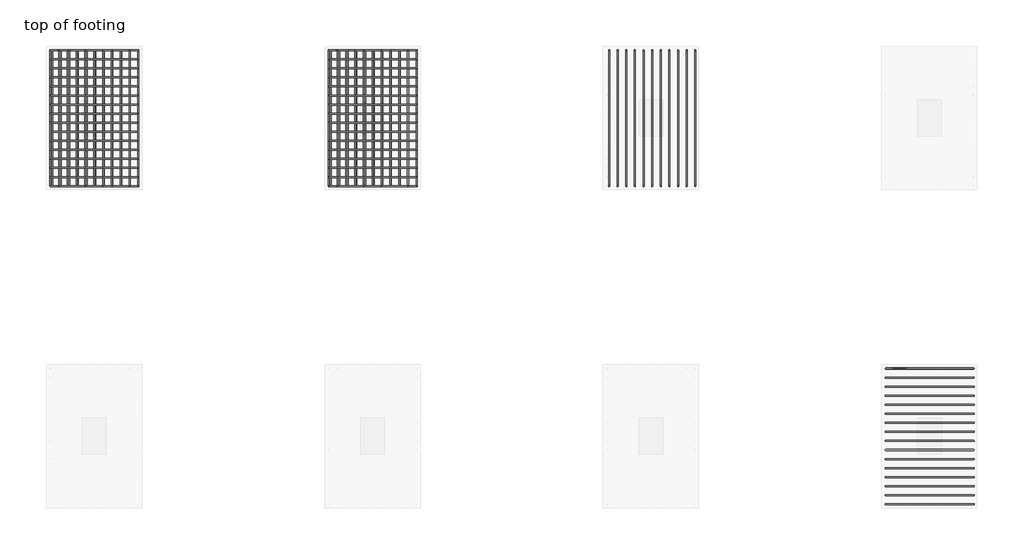
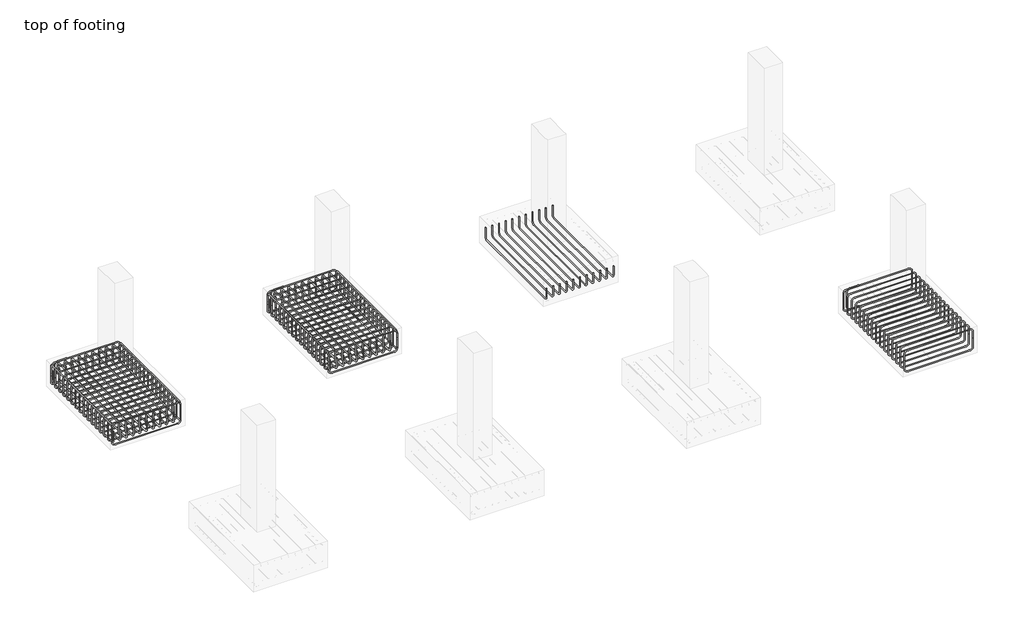
# One storey, part 6 of 8: 14 reinforcing bars.
"""IFC4 building model written with IfcOpenShell, lengths in millimetres."""

from ifc_helpers import new_model, si_unit, point, frame, origin, place, context, project, spatial, polyline, circle_curve, trimmed, segment, composite_curve, source, transform, mapped, element, save
from ifc_brep_helpers import swept_disk

model = new_model("IFC4")

# Units and contexts
model_context = context("Model", 3, world=origin())
ifc_project = project(units=[si_unit("LENGTHUNIT", "METRE", prefix="MILLI")], contexts=[model_context])

# Site, building, storey
site = spatial("IfcSite", under=ifc_project)
building = spatial("IfcBuilding", under=site)
storey = spatial("IfcBuildingStorey", under=building, Name="top of footing", Elevation=-1828.8)

# Reinforcing bars
placement = place(None, origin())
reinforcing_bar_shape = source(origin(), model_context, "Body", "SolidModel", [
    swept_disk(composite_curve([segment(polyline([(-10685.4300189, 16682.8075251, -2014.4920065), (-10685.4300189, 16682.8075251, -2161.7920065)]), True, "CONTINUOUS"), segment(trimmed(circle_curve(frame((-10685.4300189, 16729.1575251, -2161.7920065), z_axis=(1.0, 0.0, 0.0), x_axis=(0.0, -46.349999999998545, 0.0)), 46.35), [point((-10685.4300189, 16682.8075251, -2161.7920065))], [point((-10685.4300189, 16729.1575251, -2208.1420065))], True, "CARTESIAN"), True, "CONTINUOUS"), segment(polyline([(-10685.4300189, 16729.1575251, -2208.1420065), (-10685.4300189, 18343.7575251, -2208.1420065)]), True, "CONTINUOUS"), segment(trimmed(circle_curve(frame((-10685.4300189, 18343.7575251, -2161.7920065), z_axis=(1.0, 0.0, 0.0), x_axis=(0.0, 0.0, -46.350000000000364)), 46.35), [point((-10685.4300189, 18343.7575251, -2208.1420065))], [point((-10685.4300189, 18390.1075251, -2161.7920065))], True, "CARTESIAN"), True, "CONTINUOUS"), segment(polyline([(-10685.4300189, 18390.1075251, -2161.7920065), (-10685.4300189, 18390.1075251, -2014.4920065)]), True, "CONTINUOUS")], self_intersect=False), 6.35),
])
element("IfcReinforcingBar", 1, at=placement, inside=storey, context=model_context, shape_type="MappedRepresentation", body=[
    mapped(reinforcing_bar_shape, transform((0.0, 0.0, 0.0), x_axis=(1.0, 0.0, 0.0), y_axis=(0.0, 1.0, 0.0), z_axis=(0.0, 0.0, 1.0))),
    mapped(reinforcing_bar_shape, transform((-108.3645139, 0.0, 0.0), x_axis=(1.0, 0.0, 0.0), y_axis=(0.0, 1.0, 0.0), z_axis=(0.0, 0.0, 1.0))),
    mapped(reinforcing_bar_shape, transform((-216.7290279, 0.0, 0.0), x_axis=(1.0, 0.0, 0.0), y_axis=(0.0, 1.0, 0.0), z_axis=(0.0, 0.0, 1.0))),
    mapped(reinforcing_bar_shape, transform((-325.0935418, 0.0, 0.0), x_axis=(1.0, 0.0, 0.0), y_axis=(0.0, 1.0, 0.0), z_axis=(0.0, 0.0, 1.0))),
    mapped(reinforcing_bar_shape, transform((-433.4580557, 0.0, 0.0), x_axis=(1.0, 0.0, 0.0), y_axis=(0.0, 1.0, 0.0), z_axis=(0.0, 0.0, 1.0))),
    mapped(reinforcing_bar_shape, transform((-541.8225696, 0.0, 0.0), x_axis=(1.0, 0.0, 0.0), y_axis=(0.0, 1.0, 0.0), z_axis=(0.0, 0.0, 1.0))),
    mapped(reinforcing_bar_shape, transform((-650.1870836, 0.0, 0.0), x_axis=(1.0, 0.0, 0.0), y_axis=(0.0, 1.0, 0.0), z_axis=(0.0, 0.0, 1.0))),
    mapped(reinforcing_bar_shape, transform((-758.5515975, 0.0, 0.0), x_axis=(1.0, 0.0, 0.0), y_axis=(0.0, 1.0, 0.0), z_axis=(0.0, 0.0, 1.0))),
    mapped(reinforcing_bar_shape, transform((-866.9161114, 0.0, 0.0), x_axis=(1.0, 0.0, 0.0), y_axis=(0.0, 1.0, 0.0), z_axis=(0.0, 0.0, 1.0))),
    mapped(reinforcing_bar_shape, transform((-975.2806253, 0.0, 0.0), x_axis=(1.0, 0.0, 0.0), y_axis=(0.0, 1.0, 0.0), z_axis=(0.0, 0.0, 1.0))),
    mapped(reinforcing_bar_shape, transform((-1083.6451393, 0.0, 0.0), x_axis=(1.0, 0.0, 0.0), y_axis=(0.0, 1.0, 0.0), z_axis=(0.0, 0.0, 1.0))),
])
reinforcing_bar_2_shape = source(origin(), model_context, "Body", "SolidModel", [
    swept_disk(composite_curve([segment(polyline([(-11792.7300189, 16682.8075251, -2085.8010212), (-11792.7300189, 16682.8075251, -1938.5010212)]), True, "CONTINUOUS"), segment(trimmed(circle_curve(frame((-11792.7300189, 16729.1575251, -1938.5010212), z_axis=(-1.0, 0.0, 0.0), x_axis=(0.0, -46.349999999998545, 0.0)), 46.35), [point((-11792.7300189, 16682.8075251, -1938.5010212))], [point((-11792.7300189, 16729.1575251, -1892.1510212))], True, "CARTESIAN"), True, "CONTINUOUS"), segment(polyline([(-11792.7300189, 16729.1575251, -1892.1510212), (-11792.7300189, 18343.7575251, -1892.1510212)]), True, "CONTINUOUS"), segment(trimmed(circle_curve(frame((-11792.7300189, 18343.7575251, -1938.5010212), z_axis=(-1.0, 0.0, 0.0), x_axis=(0.0, 0.0, 46.34999999999991)), 46.35), [point((-11792.7300189, 18343.7575251, -1892.1510212))], [point((-11792.7300189, 18390.1075251, -1938.5010212))], True, "CARTESIAN"), True, "CONTINUOUS"), segment(polyline([(-11792.7300189, 18390.1075251, -1938.5010212), (-11792.7300189, 18390.1075251, -2085.8010212)]), True, "CONTINUOUS")], self_intersect=False), 6.35),
])
element("IfcReinforcingBar", 2, at=placement, inside=storey, context=model_context, shape_type="MappedRepresentation", body=[
    mapped(reinforcing_bar_2_shape, transform((0.0, 0.0, 0.0), x_axis=(1.0, 0.0, 0.0), y_axis=(0.0, 1.0, 0.0), z_axis=(0.0, 0.0, 1.0))),
    mapped(reinforcing_bar_2_shape, transform((110.73, 0.0, 0.0), x_axis=(1.0, 0.0, 0.0), y_axis=(0.0, 1.0, 0.0), z_axis=(0.0, 0.0, 1.0))),
    mapped(reinforcing_bar_2_shape, transform((221.46, 0.0, 0.0), x_axis=(1.0, 0.0, 0.0), y_axis=(0.0, 1.0, 0.0), z_axis=(0.0, 0.0, 1.0))),
    mapped(reinforcing_bar_2_shape, transform((332.19, 0.0, 0.0), x_axis=(1.0, 0.0, 0.0), y_axis=(0.0, 1.0, 0.0), z_axis=(0.0, 0.0, 1.0))),
    mapped(reinforcing_bar_2_shape, transform((442.92, 0.0, 0.0), x_axis=(1.0, 0.0, 0.0), y_axis=(0.0, 1.0, 0.0), z_axis=(0.0, 0.0, 1.0))),
    mapped(reinforcing_bar_2_shape, transform((553.65, 0.0, 0.0), x_axis=(1.0, 0.0, 0.0), y_axis=(0.0, 1.0, 0.0), z_axis=(0.0, 0.0, 1.0))),
    mapped(reinforcing_bar_2_shape, transform((664.38, 0.0, 0.0), x_axis=(1.0, 0.0, 0.0), y_axis=(0.0, 1.0, 0.0), z_axis=(0.0, 0.0, 1.0))),
    mapped(reinforcing_bar_2_shape, transform((775.11, 0.0, 0.0), x_axis=(1.0, 0.0, 0.0), y_axis=(0.0, 1.0, 0.0), z_axis=(0.0, 0.0, 1.0))),
    mapped(reinforcing_bar_2_shape, transform((885.84, 0.0, 0.0), x_axis=(1.0, 0.0, 0.0), y_axis=(0.0, 1.0, 0.0), z_axis=(0.0, 0.0, 1.0))),
    mapped(reinforcing_bar_2_shape, transform((996.57, 0.0, 0.0), x_axis=(1.0, 0.0, 0.0), y_axis=(0.0, 1.0, 0.0), z_axis=(0.0, 0.0, 1.0))),
    mapped(reinforcing_bar_2_shape, transform((1107.3, 0.0, 0.0), x_axis=(1.0, 0.0, 0.0), y_axis=(0.0, 1.0, 0.0), z_axis=(0.0, 0.0, 1.0))),
])
element("IfcReinforcingBar", 3, at=placement, inside=storey, context=model_context, shape_type="SolidModel", body=[
    swept_disk(composite_curve([segment(polyline([(-11543.0309105, 18390.1075251, -2232.45), (-11690.3309105, 18390.1075251, -2232.45)]), True, "CONTINUOUS"), segment(trimmed(circle_curve(frame((-11690.3309105, 18390.1075251, -2186.1), z_axis=(0.0, 1.0, 0.0), x_axis=(0.0, 0.0, -46.34999999999991)), 46.35), [point((-11690.3309105, 18390.1075251, -2232.45))], [point((-11736.6809105, 18390.1075251, -2186.1))], True, "CARTESIAN"), True, "CONTINUOUS"), segment(polyline([(-11736.6809105, 18390.1075251, -2186.1), (-11736.6809105, 18390.1075251, -1921.5)]), True, "CONTINUOUS"), segment(trimmed(circle_curve(frame((-11690.3309105, 18390.1075251, -1921.5), z_axis=(0.0, 1.0, 0.0), x_axis=(-46.349999999998545, 0.0, 0.0)), 46.35), [point((-11736.6809105, 18390.1075251, -1921.5))], [point((-11690.3309105, 18390.1075251, -1875.15))], True, "CARTESIAN"), True, "CONTINUOUS"), segment(polyline([(-11690.3309105, 18390.1075251, -1875.15), (-11543.0309105, 18390.1075251, -1875.15)]), True, "CONTINUOUS")], self_intersect=False), 6.35),
])
reinforcing_bar_3_shape = source(origin(), model_context, "Body", "SolidModel", [
    swept_disk(composite_curve([segment(polyline([(-10685.4300189, 18390.1075251, -2044.8290141), (-10685.4300189, 18390.1075251, -2192.1290141)]), True, "CONTINUOUS"), segment(trimmed(circle_curve(frame((-10731.7800189, 18390.1075251, -2192.1290141), z_axis=(0.0, 1.0, 0.0), x_axis=(46.350000000000364, 0.0, 0.0)), 46.35), [point((-10685.4300189, 18390.1075251, -2192.1290141))], [point((-10731.7800189, 18390.1075251, -2238.4790141))], True, "CARTESIAN"), True, "CONTINUOUS"), segment(polyline([(-10731.7800189, 18390.1075251, -2238.4790141), (-11746.3800189, 18390.1075251, -2238.4790141)]), True, "CONTINUOUS"), segment(trimmed(circle_curve(frame((-11746.3800189, 18390.1075251, -2192.1290141), z_axis=(0.0, 1.0, 0.0), x_axis=(0.0, 0.0, -46.34999999999991)), 46.35), [point((-11746.3800189, 18390.1075251, -2238.4790141))], [point((-11792.7300189, 18390.1075251, -2192.1290141))], True, "CARTESIAN"), True, "CONTINUOUS"), segment(polyline([(-11792.7300189, 18390.1075251, -2192.1290141), (-11792.7300189, 18390.1075251, -2044.8290141)]), True, "CONTINUOUS")], self_intersect=False), 6.35),
])
element("IfcReinforcingBar", 4, at=placement, inside=storey, context=model_context, shape_type="MappedRepresentation", body=[
    mapped(reinforcing_bar_3_shape, transform((0.0, 0.0, 0.0), x_axis=(1.0, 0.0, 0.0), y_axis=(0.0, 1.0, 0.0), z_axis=(0.0, 0.0, 1.0))),
    mapped(reinforcing_bar_3_shape, transform((0.0, -113.82, 0.0), x_axis=(1.0, 0.0, 0.0), y_axis=(0.0, 1.0, 0.0), z_axis=(0.0, 0.0, 1.0))),
    mapped(reinforcing_bar_3_shape, transform((0.0, -227.64, 0.0), x_axis=(1.0, 0.0, 0.0), y_axis=(0.0, 1.0, 0.0), z_axis=(0.0, 0.0, 1.0))),
    mapped(reinforcing_bar_3_shape, transform((0.0, -341.46, 0.0), x_axis=(1.0, 0.0, 0.0), y_axis=(0.0, 1.0, 0.0), z_axis=(0.0, 0.0, 1.0))),
    mapped(reinforcing_bar_3_shape, transform((0.0, -455.28, 0.0), x_axis=(1.0, 0.0, 0.0), y_axis=(0.0, 1.0, 0.0), z_axis=(0.0, 0.0, 1.0))),
    mapped(reinforcing_bar_3_shape, transform((0.0, -569.1, 0.0), x_axis=(1.0, 0.0, 0.0), y_axis=(0.0, 1.0, 0.0), z_axis=(0.0, 0.0, 1.0))),
    mapped(reinforcing_bar_3_shape, transform((0.0, -682.92, 0.0), x_axis=(1.0, 0.0, 0.0), y_axis=(0.0, 1.0, 0.0), z_axis=(0.0, 0.0, 1.0))),
    mapped(reinforcing_bar_3_shape, transform((0.0, -796.74, 0.0), x_axis=(1.0, 0.0, 0.0), y_axis=(0.0, 1.0, 0.0), z_axis=(0.0, 0.0, 1.0))),
    mapped(reinforcing_bar_3_shape, transform((0.0, -910.56, 0.0), x_axis=(1.0, 0.0, 0.0), y_axis=(0.0, 1.0, 0.0), z_axis=(0.0, 0.0, 1.0))),
    mapped(reinforcing_bar_3_shape, transform((0.0, -1024.38, 0.0), x_axis=(1.0, 0.0, 0.0), y_axis=(0.0, 1.0, 0.0), z_axis=(0.0, 0.0, 1.0))),
    mapped(reinforcing_bar_3_shape, transform((0.0, -1138.2, 0.0), x_axis=(1.0, 0.0, 0.0), y_axis=(0.0, 1.0, 0.0), z_axis=(0.0, 0.0, 1.0))),
    mapped(reinforcing_bar_3_shape, transform((0.0, -1252.02, 0.0), x_axis=(1.0, 0.0, 0.0), y_axis=(0.0, 1.0, 0.0), z_axis=(0.0, 0.0, 1.0))),
    mapped(reinforcing_bar_3_shape, transform((0.0, -1365.84, 0.0), x_axis=(1.0, 0.0, 0.0), y_axis=(0.0, 1.0, 0.0), z_axis=(0.0, 0.0, 1.0))),
    mapped(reinforcing_bar_3_shape, transform((0.0, -1479.66, 0.0), x_axis=(1.0, 0.0, 0.0), y_axis=(0.0, 1.0, 0.0), z_axis=(0.0, 0.0, 1.0))),
    mapped(reinforcing_bar_3_shape, transform((0.0, -1593.48, 0.0), x_axis=(1.0, 0.0, 0.0), y_axis=(0.0, 1.0, 0.0), z_axis=(0.0, 0.0, 1.0))),
    mapped(reinforcing_bar_3_shape, transform((0.0, -1707.3, 0.0), x_axis=(1.0, 0.0, 0.0), y_axis=(0.0, 1.0, 0.0), z_axis=(0.0, 0.0, 1.0))),
])
reinforcing_bar_4_shape = source(origin(), model_context, "Body", "SolidModel", [
    swept_disk(composite_curve([segment(polyline([(-11792.7300189, 18390.1075251, -2075.0801535), (-11792.7300189, 18390.1075251, -1927.7801535)]), True, "CONTINUOUS"), segment(trimmed(circle_curve(frame((-11746.3800189, 18390.1075251, -1927.7801535), z_axis=(0.0, 1.0, 0.0), x_axis=(-46.350000000000364, 0.0, 0.0)), 46.35), [point((-11792.7300189, 18390.1075251, -1927.7801535))], [point((-11746.3800189, 18390.1075251, -1881.4301535))], True, "CARTESIAN"), True, "CONTINUOUS"), segment(polyline([(-11746.3800189, 18390.1075251, -1881.4301535), (-10731.7800189, 18390.1075251, -1881.4301535)]), True, "CONTINUOUS"), segment(trimmed(circle_curve(frame((-10731.7800189, 18390.1075251, -1927.7801535), z_axis=(0.0, 1.0, 0.0), x_axis=(0.0, 0.0, 46.350000000000136)), 46.35), [point((-10731.7800189, 18390.1075251, -1881.4301535))], [point((-10685.4300189, 18390.1075251, -1927.7801535))], True, "CARTESIAN"), True, "CONTINUOUS"), segment(polyline([(-10685.4300189, 18390.1075251, -1927.7801535), (-10685.4300189, 18390.1075251, -2075.0801535)]), True, "CONTINUOUS")], self_intersect=False), 6.35),
])
element("IfcReinforcingBar", 5, at=placement, inside=storey, context=model_context, shape_type="MappedRepresentation", body=[
    mapped(reinforcing_bar_4_shape, transform((0.0, 0.0, 0.0), x_axis=(1.0, 0.0, 0.0), y_axis=(0.0, 1.0, 0.0), z_axis=(0.0, 0.0, 1.0))),
    mapped(reinforcing_bar_4_shape, transform((0.0, -113.82, 0.0), x_axis=(1.0, 0.0, 0.0), y_axis=(0.0, 1.0, 0.0), z_axis=(0.0, 0.0, 1.0))),
    mapped(reinforcing_bar_4_shape, transform((0.0, -227.64, 0.0), x_axis=(1.0, 0.0, 0.0), y_axis=(0.0, 1.0, 0.0), z_axis=(0.0, 0.0, 1.0))),
    mapped(reinforcing_bar_4_shape, transform((0.0, -341.46, 0.0), x_axis=(1.0, 0.0, 0.0), y_axis=(0.0, 1.0, 0.0), z_axis=(0.0, 0.0, 1.0))),
    mapped(reinforcing_bar_4_shape, transform((0.0, -455.28, 0.0), x_axis=(1.0, 0.0, 0.0), y_axis=(0.0, 1.0, 0.0), z_axis=(0.0, 0.0, 1.0))),
    mapped(reinforcing_bar_4_shape, transform((0.0, -569.1, 0.0), x_axis=(1.0, 0.0, 0.0), y_axis=(0.0, 1.0, 0.0), z_axis=(0.0, 0.0, 1.0))),
    mapped(reinforcing_bar_4_shape, transform((0.0, -682.92, 0.0), x_axis=(1.0, 0.0, 0.0), y_axis=(0.0, 1.0, 0.0), z_axis=(0.0, 0.0, 1.0))),
    mapped(reinforcing_bar_4_shape, transform((0.0, -796.74, 0.0), x_axis=(1.0, 0.0, 0.0), y_axis=(0.0, 1.0, 0.0), z_axis=(0.0, 0.0, 1.0))),
    mapped(reinforcing_bar_4_shape, transform((0.0, -910.56, 0.0), x_axis=(1.0, 0.0, 0.0), y_axis=(0.0, 1.0, 0.0), z_axis=(0.0, 0.0, 1.0))),
    mapped(reinforcing_bar_4_shape, transform((0.0, -1024.38, 0.0), x_axis=(1.0, 0.0, 0.0), y_axis=(0.0, 1.0, 0.0), z_axis=(0.0, 0.0, 1.0))),
    mapped(reinforcing_bar_4_shape, transform((0.0, -1138.2, 0.0), x_axis=(1.0, 0.0, 0.0), y_axis=(0.0, 1.0, 0.0), z_axis=(0.0, 0.0, 1.0))),
    mapped(reinforcing_bar_4_shape, transform((0.0, -1252.02, 0.0), x_axis=(1.0, 0.0, 0.0), y_axis=(0.0, 1.0, 0.0), z_axis=(0.0, 0.0, 1.0))),
    mapped(reinforcing_bar_4_shape, transform((0.0, -1365.84, 0.0), x_axis=(1.0, 0.0, 0.0), y_axis=(0.0, 1.0, 0.0), z_axis=(0.0, 0.0, 1.0))),
    mapped(reinforcing_bar_4_shape, transform((0.0, -1479.66, 0.0), x_axis=(1.0, 0.0, 0.0), y_axis=(0.0, 1.0, 0.0), z_axis=(0.0, 0.0, 1.0))),
    mapped(reinforcing_bar_4_shape, transform((0.0, -1593.48, 0.0), x_axis=(1.0, 0.0, 0.0), y_axis=(0.0, 1.0, 0.0), z_axis=(0.0, 0.0, 1.0))),
    mapped(reinforcing_bar_4_shape, transform((0.0, -1707.3, 0.0), x_axis=(1.0, 0.0, 0.0), y_axis=(0.0, 1.0, 0.0), z_axis=(0.0, 0.0, 1.0))),
])
reinforcing_bar_5_shape = source(origin(), model_context, "Body", "SolidModel", [
    swept_disk(composite_curve([segment(polyline([(-7185.4300189, 16682.8075251, -2014.4920065), (-7185.4300189, 16682.8075251, -2161.7920065)]), True, "CONTINUOUS"), segment(trimmed(circle_curve(frame((-7185.4300189, 16729.1575251, -2161.7920065), z_axis=(1.0, 0.0, 0.0), x_axis=(0.0, -46.349999999998545, 0.0)), 46.35), [point((-7185.4300189, 16682.8075251, -2161.7920065))], [point((-7185.4300189, 16729.1575251, -2208.1420065))], True, "CARTESIAN"), True, "CONTINUOUS"), segment(polyline([(-7185.4300189, 16729.1575251, -2208.1420065), (-7185.4300189, 18343.7575251, -2208.1420065)]), True, "CONTINUOUS"), segment(trimmed(circle_curve(frame((-7185.4300189, 18343.7575251, -2161.7920065), z_axis=(1.0, 0.0, 0.0), x_axis=(0.0, 0.0, -46.350000000000364)), 46.35), [point((-7185.4300189, 18343.7575251, -2208.1420065))], [point((-7185.4300189, 18390.1075251, -2161.7920065))], True, "CARTESIAN"), True, "CONTINUOUS"), segment(polyline([(-7185.4300189, 18390.1075251, -2161.7920065), (-7185.4300189, 18390.1075251, -2014.4920065)]), True, "CONTINUOUS")], self_intersect=False), 6.35),
])
element("IfcReinforcingBar", 6, at=placement, inside=storey, context=model_context, shape_type="MappedRepresentation", body=[
    mapped(reinforcing_bar_5_shape, transform((0.0, 0.0, 0.0), x_axis=(1.0, 0.0, 0.0), y_axis=(0.0, 1.0, 0.0), z_axis=(0.0, 0.0, 1.0))),
    mapped(reinforcing_bar_5_shape, transform((-108.3645139, 0.0, 0.0), x_axis=(1.0, 0.0, 0.0), y_axis=(0.0, 1.0, 0.0), z_axis=(0.0, 0.0, 1.0))),
    mapped(reinforcing_bar_5_shape, transform((-216.7290279, 0.0, 0.0), x_axis=(1.0, 0.0, 0.0), y_axis=(0.0, 1.0, 0.0), z_axis=(0.0, 0.0, 1.0))),
    mapped(reinforcing_bar_5_shape, transform((-325.0935418, 0.0, 0.0), x_axis=(1.0, 0.0, 0.0), y_axis=(0.0, 1.0, 0.0), z_axis=(0.0, 0.0, 1.0))),
    mapped(reinforcing_bar_5_shape, transform((-433.4580557, 0.0, 0.0), x_axis=(1.0, 0.0, 0.0), y_axis=(0.0, 1.0, 0.0), z_axis=(0.0, 0.0, 1.0))),
    mapped(reinforcing_bar_5_shape, transform((-541.8225696, 0.0, 0.0), x_axis=(1.0, 0.0, 0.0), y_axis=(0.0, 1.0, 0.0), z_axis=(0.0, 0.0, 1.0))),
    mapped(reinforcing_bar_5_shape, transform((-650.1870836, 0.0, 0.0), x_axis=(1.0, 0.0, 0.0), y_axis=(0.0, 1.0, 0.0), z_axis=(0.0, 0.0, 1.0))),
    mapped(reinforcing_bar_5_shape, transform((-758.5515975, 0.0, 0.0), x_axis=(1.0, 0.0, 0.0), y_axis=(0.0, 1.0, 0.0), z_axis=(0.0, 0.0, 1.0))),
    mapped(reinforcing_bar_5_shape, transform((-866.9161114, 0.0, 0.0), x_axis=(1.0, 0.0, 0.0), y_axis=(0.0, 1.0, 0.0), z_axis=(0.0, 0.0, 1.0))),
    mapped(reinforcing_bar_5_shape, transform((-975.2806253, 0.0, 0.0), x_axis=(1.0, 0.0, 0.0), y_axis=(0.0, 1.0, 0.0), z_axis=(0.0, 0.0, 1.0))),
    mapped(reinforcing_bar_5_shape, transform((-1083.6451393, 0.0, 0.0), x_axis=(1.0, 0.0, 0.0), y_axis=(0.0, 1.0, 0.0), z_axis=(0.0, 0.0, 1.0))),
])
reinforcing_bar_6_shape = source(origin(), model_context, "Body", "SolidModel", [
    swept_disk(composite_curve([segment(polyline([(-8292.7300189, 16682.8075251, -2085.8010212), (-8292.7300189, 16682.8075251, -1938.5010212)]), True, "CONTINUOUS"), segment(trimmed(circle_curve(frame((-8292.7300189, 16729.1575251, -1938.5010212), z_axis=(-1.0, 0.0, 0.0), x_axis=(0.0, -46.349999999998545, 0.0)), 46.35), [point((-8292.7300189, 16682.8075251, -1938.5010212))], [point((-8292.7300189, 16729.1575251, -1892.1510212))], True, "CARTESIAN"), True, "CONTINUOUS"), segment(polyline([(-8292.7300189, 16729.1575251, -1892.1510212), (-8292.7300189, 18343.7575251, -1892.1510212)]), True, "CONTINUOUS"), segment(trimmed(circle_curve(frame((-8292.7300189, 18343.7575251, -1938.5010212), z_axis=(-1.0, 0.0, 0.0), x_axis=(0.0, 0.0, 46.34999999999991)), 46.35), [point((-8292.7300189, 18343.7575251, -1892.1510212))], [point((-8292.7300189, 18390.1075251, -1938.5010212))], True, "CARTESIAN"), True, "CONTINUOUS"), segment(polyline([(-8292.7300189, 18390.1075251, -1938.5010212), (-8292.7300189, 18390.1075251, -2085.8010212)]), True, "CONTINUOUS")], self_intersect=False), 6.35),
])
element("IfcReinforcingBar", 7, at=placement, inside=storey, context=model_context, shape_type="MappedRepresentation", body=[
    mapped(reinforcing_bar_6_shape, transform((0.0, 0.0, 0.0), x_axis=(1.0, 0.0, 0.0), y_axis=(0.0, 1.0, 0.0), z_axis=(0.0, 0.0, 1.0))),
    mapped(reinforcing_bar_6_shape, transform((110.73, 0.0, 0.0), x_axis=(1.0, 0.0, 0.0), y_axis=(0.0, 1.0, 0.0), z_axis=(0.0, 0.0, 1.0))),
    mapped(reinforcing_bar_6_shape, transform((221.46, 0.0, 0.0), x_axis=(1.0, 0.0, 0.0), y_axis=(0.0, 1.0, 0.0), z_axis=(0.0, 0.0, 1.0))),
    mapped(reinforcing_bar_6_shape, transform((332.19, 0.0, 0.0), x_axis=(1.0, 0.0, 0.0), y_axis=(0.0, 1.0, 0.0), z_axis=(0.0, 0.0, 1.0))),
    mapped(reinforcing_bar_6_shape, transform((442.92, 0.0, 0.0), x_axis=(1.0, 0.0, 0.0), y_axis=(0.0, 1.0, 0.0), z_axis=(0.0, 0.0, 1.0))),
    mapped(reinforcing_bar_6_shape, transform((553.65, 0.0, 0.0), x_axis=(1.0, 0.0, 0.0), y_axis=(0.0, 1.0, 0.0), z_axis=(0.0, 0.0, 1.0))),
    mapped(reinforcing_bar_6_shape, transform((664.38, 0.0, 0.0), x_axis=(1.0, 0.0, 0.0), y_axis=(0.0, 1.0, 0.0), z_axis=(0.0, 0.0, 1.0))),
    mapped(reinforcing_bar_6_shape, transform((775.11, 0.0, 0.0), x_axis=(1.0, 0.0, 0.0), y_axis=(0.0, 1.0, 0.0), z_axis=(0.0, 0.0, 1.0))),
    mapped(reinforcing_bar_6_shape, transform((885.84, 0.0, 0.0), x_axis=(1.0, 0.0, 0.0), y_axis=(0.0, 1.0, 0.0), z_axis=(0.0, 0.0, 1.0))),
    mapped(reinforcing_bar_6_shape, transform((996.57, 0.0, 0.0), x_axis=(1.0, 0.0, 0.0), y_axis=(0.0, 1.0, 0.0), z_axis=(0.0, 0.0, 1.0))),
    mapped(reinforcing_bar_6_shape, transform((1107.3, 0.0, 0.0), x_axis=(1.0, 0.0, 0.0), y_axis=(0.0, 1.0, 0.0), z_axis=(0.0, 0.0, 1.0))),
])
element("IfcReinforcingBar", 8, at=placement, inside=storey, context=model_context, shape_type="SolidModel", body=[
    swept_disk(composite_curve([segment(polyline([(-8043.0309105, 18390.1075251, -2232.45), (-8190.3309105, 18390.1075251, -2232.45)]), True, "CONTINUOUS"), segment(trimmed(circle_curve(frame((-8190.3309105, 18390.1075251, -2186.1), z_axis=(0.0, 1.0, 0.0), x_axis=(0.0, 0.0, -46.34999999999991)), 46.35), [point((-8190.3309105, 18390.1075251, -2232.45))], [point((-8236.6809105, 18390.1075251, -2186.1))], True, "CARTESIAN"), True, "CONTINUOUS"), segment(polyline([(-8236.6809105, 18390.1075251, -2186.1), (-8236.6809105, 18390.1075251, -1921.5)]), True, "CONTINUOUS"), segment(trimmed(circle_curve(frame((-8190.3309105, 18390.1075251, -1921.5), z_axis=(0.0, 1.0, 0.0), x_axis=(-46.349999999999454, 0.0, 0.0)), 46.35), [point((-8236.6809105, 18390.1075251, -1921.5))], [point((-8190.3309105, 18390.1075251, -1875.15))], True, "CARTESIAN"), True, "CONTINUOUS"), segment(polyline([(-8190.3309105, 18390.1075251, -1875.15), (-8043.0309105, 18390.1075251, -1875.15)]), True, "CONTINUOUS")], self_intersect=False), 6.35),
])
reinforcing_bar_7_shape = source(origin(), model_context, "Body", "SolidModel", [
    swept_disk(composite_curve([segment(polyline([(-7185.4300189, 18390.1075251, -2044.8290141), (-7185.4300189, 18390.1075251, -2192.1290141)]), True, "CONTINUOUS"), segment(trimmed(circle_curve(frame((-7231.7800189, 18390.1075251, -2192.1290141), z_axis=(0.0, 1.0, 0.0), x_axis=(46.350000000000364, 0.0, 0.0)), 46.35), [point((-7185.4300189, 18390.1075251, -2192.1290141))], [point((-7231.7800189, 18390.1075251, -2238.4790141))], True, "CARTESIAN"), True, "CONTINUOUS"), segment(polyline([(-7231.7800189, 18390.1075251, -2238.4790141), (-8246.3800189, 18390.1075251, -2238.4790141)]), True, "CONTINUOUS"), segment(trimmed(circle_curve(frame((-8246.3800189, 18390.1075251, -2192.1290141), z_axis=(0.0, 1.0, 0.0), x_axis=(0.0, 0.0, -46.34999999999991)), 46.35), [point((-8246.3800189, 18390.1075251, -2238.4790141))], [point((-8292.7300189, 18390.1075251, -2192.1290141))], True, "CARTESIAN"), True, "CONTINUOUS"), segment(polyline([(-8292.7300189, 18390.1075251, -2192.1290141), (-8292.7300189, 18390.1075251, -2044.8290141)]), True, "CONTINUOUS")], self_intersect=False), 6.35),
])
element("IfcReinforcingBar", 9, at=placement, inside=storey, context=model_context, shape_type="MappedRepresentation", body=[
    mapped(reinforcing_bar_7_shape, transform((0.0, 0.0, 0.0), x_axis=(1.0, 0.0, 0.0), y_axis=(0.0, 1.0, 0.0), z_axis=(0.0, 0.0, 1.0))),
    mapped(reinforcing_bar_7_shape, transform((0.0, -113.82, 0.0), x_axis=(1.0, 0.0, 0.0), y_axis=(0.0, 1.0, 0.0), z_axis=(0.0, 0.0, 1.0))),
    mapped(reinforcing_bar_7_shape, transform((0.0, -227.64, 0.0), x_axis=(1.0, 0.0, 0.0), y_axis=(0.0, 1.0, 0.0), z_axis=(0.0, 0.0, 1.0))),
    mapped(reinforcing_bar_7_shape, transform((0.0, -341.46, 0.0), x_axis=(1.0, 0.0, 0.0), y_axis=(0.0, 1.0, 0.0), z_axis=(0.0, 0.0, 1.0))),
    mapped(reinforcing_bar_7_shape, transform((0.0, -455.28, 0.0), x_axis=(1.0, 0.0, 0.0), y_axis=(0.0, 1.0, 0.0), z_axis=(0.0, 0.0, 1.0))),
    mapped(reinforcing_bar_7_shape, transform((0.0, -569.1, 0.0), x_axis=(1.0, 0.0, 0.0), y_axis=(0.0, 1.0, 0.0), z_axis=(0.0, 0.0, 1.0))),
    mapped(reinforcing_bar_7_shape, transform((0.0, -682.92, 0.0), x_axis=(1.0, 0.0, 0.0), y_axis=(0.0, 1.0, 0.0), z_axis=(0.0, 0.0, 1.0))),
    mapped(reinforcing_bar_7_shape, transform((0.0, -796.74, 0.0), x_axis=(1.0, 0.0, 0.0), y_axis=(0.0, 1.0, 0.0), z_axis=(0.0, 0.0, 1.0))),
    mapped(reinforcing_bar_7_shape, transform((0.0, -910.56, 0.0), x_axis=(1.0, 0.0, 0.0), y_axis=(0.0, 1.0, 0.0), z_axis=(0.0, 0.0, 1.0))),
    mapped(reinforcing_bar_7_shape, transform((0.0, -1024.38, 0.0), x_axis=(1.0, 0.0, 0.0), y_axis=(0.0, 1.0, 0.0), z_axis=(0.0, 0.0, 1.0))),
    mapped(reinforcing_bar_7_shape, transform((0.0, -1138.2, 0.0), x_axis=(1.0, 0.0, 0.0), y_axis=(0.0, 1.0, 0.0), z_axis=(0.0, 0.0, 1.0))),
    mapped(reinforcing_bar_7_shape, transform((0.0, -1252.02, 0.0), x_axis=(1.0, 0.0, 0.0), y_axis=(0.0, 1.0, 0.0), z_axis=(0.0, 0.0, 1.0))),
    mapped(reinforcing_bar_7_shape, transform((0.0, -1365.84, 0.0), x_axis=(1.0, 0.0, 0.0), y_axis=(0.0, 1.0, 0.0), z_axis=(0.0, 0.0, 1.0))),
    mapped(reinforcing_bar_7_shape, transform((0.0, -1479.66, 0.0), x_axis=(1.0, 0.0, 0.0), y_axis=(0.0, 1.0, 0.0), z_axis=(0.0, 0.0, 1.0))),
    mapped(reinforcing_bar_7_shape, transform((0.0, -1593.48, 0.0), x_axis=(1.0, 0.0, 0.0), y_axis=(0.0, 1.0, 0.0), z_axis=(0.0, 0.0, 1.0))),
    mapped(reinforcing_bar_7_shape, transform((0.0, -1707.3, 0.0), x_axis=(1.0, 0.0, 0.0), y_axis=(0.0, 1.0, 0.0), z_axis=(0.0, 0.0, 1.0))),
])
reinforcing_bar_8_shape = source(origin(), model_context, "Body", "SolidModel", [
    swept_disk(composite_curve([segment(polyline([(-8292.7300189, 18390.1075251, -2075.0801535), (-8292.7300189, 18390.1075251, -1927.7801535)]), True, "CONTINUOUS"), segment(trimmed(circle_curve(frame((-8246.3800189, 18390.1075251, -1927.7801535), z_axis=(0.0, 1.0, 0.0), x_axis=(-46.350000000000364, 0.0, 0.0)), 46.35), [point((-8292.7300189, 18390.1075251, -1927.7801535))], [point((-8246.3800189, 18390.1075251, -1881.4301535))], True, "CARTESIAN"), True, "CONTINUOUS"), segment(polyline([(-8246.3800189, 18390.1075251, -1881.4301535), (-7231.7800189, 18390.1075251, -1881.4301535)]), True, "CONTINUOUS"), segment(trimmed(circle_curve(frame((-7231.7800189, 18390.1075251, -1927.7801535), z_axis=(0.0, 1.0, 0.0), x_axis=(0.0, 0.0, 46.350000000000136)), 46.35), [point((-7231.7800189, 18390.1075251, -1881.4301535))], [point((-7185.4300189, 18390.1075251, -1927.7801535))], True, "CARTESIAN"), True, "CONTINUOUS"), segment(polyline([(-7185.4300189, 18390.1075251, -1927.7801535), (-7185.4300189, 18390.1075251, -2075.0801535)]), True, "CONTINUOUS")], self_intersect=False), 6.35),
])
element("IfcReinforcingBar", 10, at=placement, inside=storey, context=model_context, shape_type="MappedRepresentation", body=[
    mapped(reinforcing_bar_8_shape, transform((0.0, 0.0, 0.0), x_axis=(1.0, 0.0, 0.0), y_axis=(0.0, 1.0, 0.0), z_axis=(0.0, 0.0, 1.0))),
    mapped(reinforcing_bar_8_shape, transform((0.0, -113.82, 0.0), x_axis=(1.0, 0.0, 0.0), y_axis=(0.0, 1.0, 0.0), z_axis=(0.0, 0.0, 1.0))),
    mapped(reinforcing_bar_8_shape, transform((0.0, -227.64, 0.0), x_axis=(1.0, 0.0, 0.0), y_axis=(0.0, 1.0, 0.0), z_axis=(0.0, 0.0, 1.0))),
    mapped(reinforcing_bar_8_shape, transform((0.0, -341.46, 0.0), x_axis=(1.0, 0.0, 0.0), y_axis=(0.0, 1.0, 0.0), z_axis=(0.0, 0.0, 1.0))),
    mapped(reinforcing_bar_8_shape, transform((0.0, -455.28, 0.0), x_axis=(1.0, 0.0, 0.0), y_axis=(0.0, 1.0, 0.0), z_axis=(0.0, 0.0, 1.0))),
    mapped(reinforcing_bar_8_shape, transform((0.0, -569.1, 0.0), x_axis=(1.0, 0.0, 0.0), y_axis=(0.0, 1.0, 0.0), z_axis=(0.0, 0.0, 1.0))),
    mapped(reinforcing_bar_8_shape, transform((0.0, -682.92, 0.0), x_axis=(1.0, 0.0, 0.0), y_axis=(0.0, 1.0, 0.0), z_axis=(0.0, 0.0, 1.0))),
    mapped(reinforcing_bar_8_shape, transform((0.0, -796.74, 0.0), x_axis=(1.0, 0.0, 0.0), y_axis=(0.0, 1.0, 0.0), z_axis=(0.0, 0.0, 1.0))),
    mapped(reinforcing_bar_8_shape, transform((0.0, -910.56, 0.0), x_axis=(1.0, 0.0, 0.0), y_axis=(0.0, 1.0, 0.0), z_axis=(0.0, 0.0, 1.0))),
    mapped(reinforcing_bar_8_shape, transform((0.0, -1024.38, 0.0), x_axis=(1.0, 0.0, 0.0), y_axis=(0.0, 1.0, 0.0), z_axis=(0.0, 0.0, 1.0))),
    mapped(reinforcing_bar_8_shape, transform((0.0, -1138.2, 0.0), x_axis=(1.0, 0.0, 0.0), y_axis=(0.0, 1.0, 0.0), z_axis=(0.0, 0.0, 1.0))),
    mapped(reinforcing_bar_8_shape, transform((0.0, -1252.02, 0.0), x_axis=(1.0, 0.0, 0.0), y_axis=(0.0, 1.0, 0.0), z_axis=(0.0, 0.0, 1.0))),
    mapped(reinforcing_bar_8_shape, transform((0.0, -1365.84, 0.0), x_axis=(1.0, 0.0, 0.0), y_axis=(0.0, 1.0, 0.0), z_axis=(0.0, 0.0, 1.0))),
    mapped(reinforcing_bar_8_shape, transform((0.0, -1479.66, 0.0), x_axis=(1.0, 0.0, 0.0), y_axis=(0.0, 1.0, 0.0), z_axis=(0.0, 0.0, 1.0))),
    mapped(reinforcing_bar_8_shape, transform((0.0, -1593.48, 0.0), x_axis=(1.0, 0.0, 0.0), y_axis=(0.0, 1.0, 0.0), z_axis=(0.0, 0.0, 1.0))),
    mapped(reinforcing_bar_8_shape, transform((0.0, -1707.3, 0.0), x_axis=(1.0, 0.0, 0.0), y_axis=(0.0, 1.0, 0.0), z_axis=(0.0, 0.0, 1.0))),
])
reinforcing_bar_9_shape = source(origin(), model_context, "Body", "SolidModel", [
    swept_disk(composite_curve([segment(polyline([(-3685.4300189, 16682.8075251, -2014.4920065), (-3685.4300189, 16682.8075251, -2161.7920065)]), True, "CONTINUOUS"), segment(trimmed(circle_curve(frame((-3685.4300189, 16729.1575251, -2161.7920065), z_axis=(1.0, 0.0, 0.0), x_axis=(0.0, -46.349999999998545, 0.0)), 46.35), [point((-3685.4300189, 16682.8075251, -2161.7920065))], [point((-3685.4300189, 16729.1575251, -2208.1420065))], True, "CARTESIAN"), True, "CONTINUOUS"), segment(polyline([(-3685.4300189, 16729.1575251, -2208.1420065), (-3685.4300189, 18343.7575251, -2208.1420065)]), True, "CONTINUOUS"), segment(trimmed(circle_curve(frame((-3685.4300189, 18343.7575251, -2161.7920065), z_axis=(1.0, 0.0, 0.0), x_axis=(0.0, 0.0, -46.350000000000364)), 46.35), [point((-3685.4300189, 18343.7575251, -2208.1420065))], [point((-3685.4300189, 18390.1075251, -2161.7920065))], True, "CARTESIAN"), True, "CONTINUOUS"), segment(polyline([(-3685.4300189, 18390.1075251, -2161.7920065), (-3685.4300189, 18390.1075251, -2014.4920065)]), True, "CONTINUOUS")], self_intersect=False), 6.35),
])
element("IfcReinforcingBar", 11, at=placement, inside=storey, context=model_context, shape_type="MappedRepresentation", body=[
    mapped(reinforcing_bar_9_shape, transform((0.0, 0.0, 0.0), x_axis=(1.0, 0.0, 0.0), y_axis=(0.0, 1.0, 0.0), z_axis=(0.0, 0.0, 1.0))),
    mapped(reinforcing_bar_9_shape, transform((-108.3645139, 0.0, 0.0), x_axis=(1.0, 0.0, 0.0), y_axis=(0.0, 1.0, 0.0), z_axis=(0.0, 0.0, 1.0))),
    mapped(reinforcing_bar_9_shape, transform((-216.7290279, 0.0, 0.0), x_axis=(1.0, 0.0, 0.0), y_axis=(0.0, 1.0, 0.0), z_axis=(0.0, 0.0, 1.0))),
    mapped(reinforcing_bar_9_shape, transform((-325.0935418, 0.0, 0.0), x_axis=(1.0, 0.0, 0.0), y_axis=(0.0, 1.0, 0.0), z_axis=(0.0, 0.0, 1.0))),
    mapped(reinforcing_bar_9_shape, transform((-433.4580557, 0.0, 0.0), x_axis=(1.0, 0.0, 0.0), y_axis=(0.0, 1.0, 0.0), z_axis=(0.0, 0.0, 1.0))),
    mapped(reinforcing_bar_9_shape, transform((-541.8225696, 0.0, 0.0), x_axis=(1.0, 0.0, 0.0), y_axis=(0.0, 1.0, 0.0), z_axis=(0.0, 0.0, 1.0))),
    mapped(reinforcing_bar_9_shape, transform((-650.1870836, 0.0, 0.0), x_axis=(1.0, 0.0, 0.0), y_axis=(0.0, 1.0, 0.0), z_axis=(0.0, 0.0, 1.0))),
    mapped(reinforcing_bar_9_shape, transform((-758.5515975, 0.0, 0.0), x_axis=(1.0, 0.0, 0.0), y_axis=(0.0, 1.0, 0.0), z_axis=(0.0, 0.0, 1.0))),
    mapped(reinforcing_bar_9_shape, transform((-866.9161114, 0.0, 0.0), x_axis=(1.0, 0.0, 0.0), y_axis=(0.0, 1.0, 0.0), z_axis=(0.0, 0.0, 1.0))),
    mapped(reinforcing_bar_9_shape, transform((-975.2806253, 0.0, 0.0), x_axis=(1.0, 0.0, 0.0), y_axis=(0.0, 1.0, 0.0), z_axis=(0.0, 0.0, 1.0))),
    mapped(reinforcing_bar_9_shape, transform((-1083.6451393, 0.0, 0.0), x_axis=(1.0, 0.0, 0.0), y_axis=(0.0, 1.0, 0.0), z_axis=(0.0, 0.0, 1.0))),
])
element("IfcReinforcingBar", 12, at=placement, inside=storey, context=model_context, shape_type="SolidModel", body=[
    swept_disk(composite_curve([segment(polyline([(-1043.0309105, 14390.1075251, -2232.45), (-1190.3309105, 14390.1075251, -2232.45)]), True, "CONTINUOUS"), segment(trimmed(circle_curve(frame((-1190.3309105, 14390.1075251, -2186.1), z_axis=(0.0, 1.0, 0.0), x_axis=(0.0, 0.0, -46.34999999999991)), 46.35), [point((-1190.3309105, 14390.1075251, -2232.45))], [point((-1236.6809105, 14390.1075251, -2186.1))], True, "CARTESIAN"), True, "CONTINUOUS"), segment(polyline([(-1236.6809105, 14390.1075251, -2186.1), (-1236.6809105, 14390.1075251, -1921.5)]), True, "CONTINUOUS"), segment(trimmed(circle_curve(frame((-1190.3309105, 14390.1075251, -1921.5), z_axis=(0.0, 1.0, 0.0), x_axis=(-46.34999999999991, 0.0, 0.0)), 46.35), [point((-1236.6809105, 14390.1075251, -1921.5))], [point((-1190.3309105, 14390.1075251, -1875.15))], True, "CARTESIAN"), True, "CONTINUOUS"), segment(polyline([(-1190.3309105, 14390.1075251, -1875.15), (-1043.0309105, 14390.1075251, -1875.15)]), True, "CONTINUOUS")], self_intersect=False), 6.35),
])
reinforcing_bar_10_shape = source(origin(), model_context, "Body", "SolidModel", [
    swept_disk(composite_curve([segment(polyline([(-185.4300189, 14390.1075251, -2044.8290141), (-185.4300189, 14390.1075251, -2192.1290141)]), True, "CONTINUOUS"), segment(trimmed(circle_curve(frame((-231.7800189, 14390.1075251, -2192.1290141), z_axis=(0.0, 1.0, 0.0), x_axis=(46.349999999999994, 0.0, 0.0)), 46.35), [point((-185.4300189, 14390.1075251, -2192.1290141))], [point((-231.7800189, 14390.1075251, -2238.4790141))], True, "CARTESIAN"), True, "CONTINUOUS"), segment(polyline([(-231.7800189, 14390.1075251, -2238.4790141), (-1246.3800189, 14390.1075251, -2238.4790141)]), True, "CONTINUOUS"), segment(trimmed(circle_curve(frame((-1246.3800189, 14390.1075251, -2192.1290141), z_axis=(0.0, 1.0, 0.0), x_axis=(0.0, 0.0, -46.34999999999991)), 46.35), [point((-1246.3800189, 14390.1075251, -2238.4790141))], [point((-1292.7300189, 14390.1075251, -2192.1290141))], True, "CARTESIAN"), True, "CONTINUOUS"), segment(polyline([(-1292.7300189, 14390.1075251, -2192.1290141), (-1292.7300189, 14390.1075251, -2044.8290141)]), True, "CONTINUOUS")], self_intersect=False), 6.35),
])
element("IfcReinforcingBar", 13, at=placement, inside=storey, context=model_context, shape_type="MappedRepresentation", body=[
    mapped(reinforcing_bar_10_shape, transform((0.0, 0.0, 0.0), x_axis=(1.0, 0.0, 0.0), y_axis=(0.0, 1.0, 0.0), z_axis=(0.0, 0.0, 1.0))),
    mapped(reinforcing_bar_10_shape, transform((0.0, -113.82, 0.0), x_axis=(1.0, 0.0, 0.0), y_axis=(0.0, 1.0, 0.0), z_axis=(0.0, 0.0, 1.0))),
    mapped(reinforcing_bar_10_shape, transform((0.0, -227.64, 0.0), x_axis=(1.0, 0.0, 0.0), y_axis=(0.0, 1.0, 0.0), z_axis=(0.0, 0.0, 1.0))),
    mapped(reinforcing_bar_10_shape, transform((0.0, -341.46, 0.0), x_axis=(1.0, 0.0, 0.0), y_axis=(0.0, 1.0, 0.0), z_axis=(0.0, 0.0, 1.0))),
    mapped(reinforcing_bar_10_shape, transform((0.0, -455.28, 0.0), x_axis=(1.0, 0.0, 0.0), y_axis=(0.0, 1.0, 0.0), z_axis=(0.0, 0.0, 1.0))),
    mapped(reinforcing_bar_10_shape, transform((0.0, -569.1, 0.0), x_axis=(1.0, 0.0, 0.0), y_axis=(0.0, 1.0, 0.0), z_axis=(0.0, 0.0, 1.0))),
    mapped(reinforcing_bar_10_shape, transform((0.0, -682.92, 0.0), x_axis=(1.0, 0.0, 0.0), y_axis=(0.0, 1.0, 0.0), z_axis=(0.0, 0.0, 1.0))),
    mapped(reinforcing_bar_10_shape, transform((0.0, -796.74, 0.0), x_axis=(1.0, 0.0, 0.0), y_axis=(0.0, 1.0, 0.0), z_axis=(0.0, 0.0, 1.0))),
    mapped(reinforcing_bar_10_shape, transform((0.0, -910.56, 0.0), x_axis=(1.0, 0.0, 0.0), y_axis=(0.0, 1.0, 0.0), z_axis=(0.0, 0.0, 1.0))),
    mapped(reinforcing_bar_10_shape, transform((0.0, -1024.38, 0.0), x_axis=(1.0, 0.0, 0.0), y_axis=(0.0, 1.0, 0.0), z_axis=(0.0, 0.0, 1.0))),
    mapped(reinforcing_bar_10_shape, transform((0.0, -1138.2, 0.0), x_axis=(1.0, 0.0, 0.0), y_axis=(0.0, 1.0, 0.0), z_axis=(0.0, 0.0, 1.0))),
    mapped(reinforcing_bar_10_shape, transform((0.0, -1252.02, 0.0), x_axis=(1.0, 0.0, 0.0), y_axis=(0.0, 1.0, 0.0), z_axis=(0.0, 0.0, 1.0))),
    mapped(reinforcing_bar_10_shape, transform((0.0, -1365.84, 0.0), x_axis=(1.0, 0.0, 0.0), y_axis=(0.0, 1.0, 0.0), z_axis=(0.0, 0.0, 1.0))),
    mapped(reinforcing_bar_10_shape, transform((0.0, -1479.66, 0.0), x_axis=(1.0, 0.0, 0.0), y_axis=(0.0, 1.0, 0.0), z_axis=(0.0, 0.0, 1.0))),
    mapped(reinforcing_bar_10_shape, transform((0.0, -1593.48, 0.0), x_axis=(1.0, 0.0, 0.0), y_axis=(0.0, 1.0, 0.0), z_axis=(0.0, 0.0, 1.0))),
    mapped(reinforcing_bar_10_shape, transform((0.0, -1707.3, 0.0), x_axis=(1.0, 0.0, 0.0), y_axis=(0.0, 1.0, 0.0), z_axis=(0.0, 0.0, 1.0))),
])
reinforcing_bar_11_shape = source(origin(), model_context, "Body", "SolidModel", [
    swept_disk(composite_curve([segment(polyline([(-1292.7300189, 14390.1075251, -2075.0801535), (-1292.7300189, 14390.1075251, -1927.7801535)]), True, "CONTINUOUS"), segment(trimmed(circle_curve(frame((-1246.3800189, 14390.1075251, -1927.7801535), z_axis=(0.0, 1.0, 0.0), x_axis=(-46.34999999999991, 0.0, 0.0)), 46.35), [point((-1292.7300189, 14390.1075251, -1927.7801535))], [point((-1246.3800189, 14390.1075251, -1881.4301535))], True, "CARTESIAN"), True, "CONTINUOUS"), segment(polyline([(-1246.3800189, 14390.1075251, -1881.4301535), (-231.7800189, 14390.1075251, -1881.4301535)]), True, "CONTINUOUS"), segment(trimmed(circle_curve(frame((-231.7800189, 14390.1075251, -1927.7801535), z_axis=(0.0, 1.0, 0.0), x_axis=(0.0, 0.0, 46.350000000000136)), 46.35), [point((-231.7800189, 14390.1075251, -1881.4301535))], [point((-185.4300189, 14390.1075251, -1927.7801535))], True, "CARTESIAN"), True, "CONTINUOUS"), segment(polyline([(-185.4300189, 14390.1075251, -1927.7801535), (-185.4300189, 14390.1075251, -2075.0801535)]), True, "CONTINUOUS")], self_intersect=False), 6.35),
])
element("IfcReinforcingBar", 14, at=placement, inside=storey, context=model_context, shape_type="MappedRepresentation", body=[
    mapped(reinforcing_bar_11_shape, transform((0.0, 0.0, 0.0), x_axis=(1.0, 0.0, 0.0), y_axis=(0.0, 1.0, 0.0), z_axis=(0.0, 0.0, 1.0))),
    mapped(reinforcing_bar_11_shape, transform((0.0, -113.82, 0.0), x_axis=(1.0, 0.0, 0.0), y_axis=(0.0, 1.0, 0.0), z_axis=(0.0, 0.0, 1.0))),
    mapped(reinforcing_bar_11_shape, transform((0.0, -227.64, 0.0), x_axis=(1.0, 0.0, 0.0), y_axis=(0.0, 1.0, 0.0), z_axis=(0.0, 0.0, 1.0))),
    mapped(reinforcing_bar_11_shape, transform((0.0, -341.46, 0.0), x_axis=(1.0, 0.0, 0.0), y_axis=(0.0, 1.0, 0.0), z_axis=(0.0, 0.0, 1.0))),
    mapped(reinforcing_bar_11_shape, transform((0.0, -455.28, 0.0), x_axis=(1.0, 0.0, 0.0), y_axis=(0.0, 1.0, 0.0), z_axis=(0.0, 0.0, 1.0))),
    mapped(reinforcing_bar_11_shape, transform((0.0, -569.1, 0.0), x_axis=(1.0, 0.0, 0.0), y_axis=(0.0, 1.0, 0.0), z_axis=(0.0, 0.0, 1.0))),
    mapped(reinforcing_bar_11_shape, transform((0.0, -682.92, 0.0), x_axis=(1.0, 0.0, 0.0), y_axis=(0.0, 1.0, 0.0), z_axis=(0.0, 0.0, 1.0))),
    mapped(reinforcing_bar_11_shape, transform((0.0, -796.74, 0.0), x_axis=(1.0, 0.0, 0.0), y_axis=(0.0, 1.0, 0.0), z_axis=(0.0, 0.0, 1.0))),
    mapped(reinforcing_bar_11_shape, transform((0.0, -910.56, 0.0), x_axis=(1.0, 0.0, 0.0), y_axis=(0.0, 1.0, 0.0), z_axis=(0.0, 0.0, 1.0))),
    mapped(reinforcing_bar_11_shape, transform((0.0, -1024.38, 0.0), x_axis=(1.0, 0.0, 0.0), y_axis=(0.0, 1.0, 0.0), z_axis=(0.0, 0.0, 1.0))),
    mapped(reinforcing_bar_11_shape, transform((0.0, -1138.2, 0.0), x_axis=(1.0, 0.0, 0.0), y_axis=(0.0, 1.0, 0.0), z_axis=(0.0, 0.0, 1.0))),
    mapped(reinforcing_bar_11_shape, transform((0.0, -1252.02, 0.0), x_axis=(1.0, 0.0, 0.0), y_axis=(0.0, 1.0, 0.0), z_axis=(0.0, 0.0, 1.0))),
    mapped(reinforcing_bar_11_shape, transform((0.0, -1365.84, 0.0), x_axis=(1.0, 0.0, 0.0), y_axis=(0.0, 1.0, 0.0), z_axis=(0.0, 0.0, 1.0))),
    mapped(reinforcing_bar_11_shape, transform((0.0, -1479.66, 0.0), x_axis=(1.0, 0.0, 0.0), y_axis=(0.0, 1.0, 0.0), z_axis=(0.0, 0.0, 1.0))),
    mapped(reinforcing_bar_11_shape, transform((0.0, -1593.48, 0.0), x_axis=(1.0, 0.0, 0.0), y_axis=(0.0, 1.0, 0.0), z_axis=(0.0, 0.0, 1.0))),
    mapped(reinforcing_bar_11_shape, transform((0.0, -1707.3, 0.0), x_axis=(1.0, 0.0, 0.0), y_axis=(0.0, 1.0, 0.0), z_axis=(0.0, 0.0, 1.0))),
])

save(model, "model.ifc")

# Revit data of these elements
# Elements 1, 2, 3, 4, 5, 6, 7, 8, 9, 10, 11, 12, 13, 14 (IfcReinforcingBar)
#   Phase Created = New Construction
